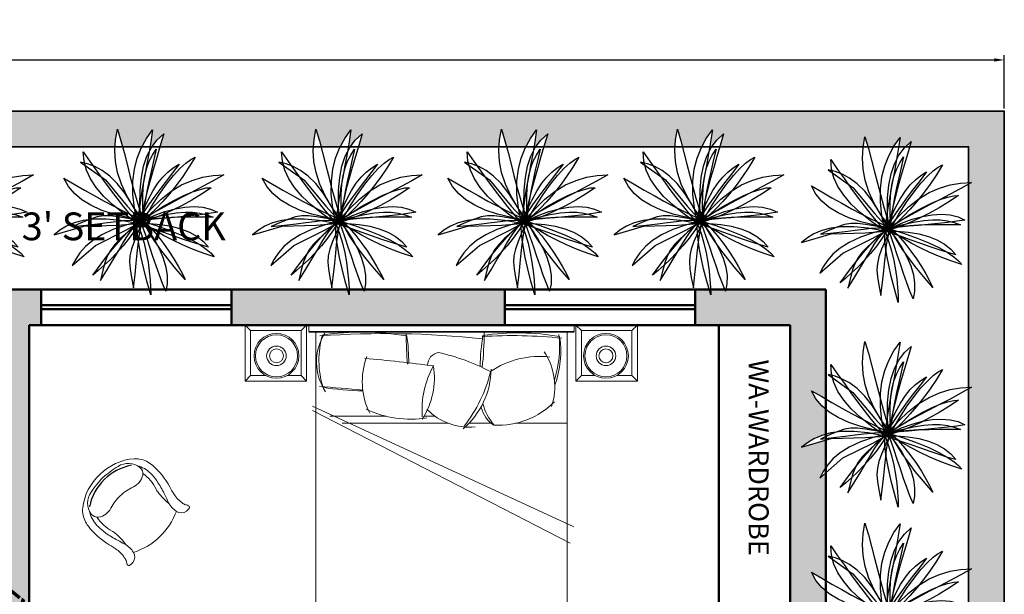
# Model space of a CAD drawing. Units: inches. Extents: x 2442 to 3851, y 589 to 2836.
# Tile 10 of 22: x 2845 to 3094, y 1880 to 2025. Entities that reach past the tile are written whole.
import ezdxf

# ---------------------------------------------------------------- set-up
doc = ezdxf.new("R2010")
doc.units = ezdxf.units.IN
for name, color, linetype, lineweight in [('0.10', 252, 'Continuous', 9), ('0.15', 34, 'Continuous', 15), ('A-ANNO-DIMS', 2, 'Continuous', 18), ('A-ANNO-TEXT', 7, 'Continuous', 18), ('A-FURN', 8, 'Continuous', 18), ('A-WALL', 7, 'Continuous', 50), ('A-WALL-PATT', 8, 'Continuous', 13), ('C-PROP', 7, 'Continuous', 35), ('L-PLNT', 94, 'Continuous', 18)]:
    doc.layers.add(name, color=color, linetype=linetype, lineweight=lineweight)
doc.layers.add('DIENHOA', color=3, linetype='Continuous')
doc.layers.add('IFF-FURN-DETAIL', color=250, linetype='Continuous')
doc.styles.get("Standard").update_dxf_attribs({"font": 'arial.ttf'})
doc.dimstyles.new('ISO-25', dxfattribs={"dimtxt": 8, "dimasz": 2.5, "dimexe": 1.25, "dimexo": 0.625, "dimtad": 1, "dimlunit": 3, "dimtxsty": 'Standard', "dimcen": 2.5, "dimadec": 0, "dimazin": 0, "dimtfac": 1, "dimtmove": 0, "dimatfit": 3, "dimfxl": 1, "dimarcsym": 0})

# ---------------------------------------------------------------- blocks, each defined once
blk = doc.blocks.new('camita')
at = {"layer": '0.10'}
for p, q in [((-0.85, -0.045), (0.85, -0.045)), ((-0.805, -0.045), (-0.805, -2.0485)), ((0.805, -0.045), (0.805, -2.0485)), ((-0.8271, -0.521), (0.8464, -1.2932)), ((-0.8271, -0.5476), (0.8236, -1.3992)), ((-0.7161, -0.585), (-0.3554, -0.585)), ((-0.638, -0.63), (0.0434, -0.63)), ((-0.1136, -0.585), (-0.0485, -0.585)), ((0.1749, -0.63), (0.3179, -0.63)), ((0.4739, -0.63), (0.805, -0.63)), ((-0.8354, -2), (0.8464, -2))]:
    blk.add_line(p, q, dxfattribs=at)
blk.add_lwpolyline([(-0.85, -0.0405), (0.85, -0.0405), (0.85, 0), (-0.85, 0)], close=True, dxfattribs=at)
for centre, radius, start, end in [((-0.4574, -0.2364), 0.3443, 147.50996, 213.83359), ((-0.3639, -5.8457), 5.7909, 83.80731, 94.12107), ((-0.5104, -1.7232), 1.6781, 80.12554, 98.66187), ((2.3534, -0.0532), 2.5803, 180.10628, 184.38541), ((-1.4396, -0.0609), 1.7117, 352.92911, 0.39592), ((0.4863, -1.6286), 1.5781, 80.16015, 98.05996), ((0.0294, -0.1377), 0.7262, 342.58415, 6.00484), ((-0.1997, -0.2266), 0.5864, 163.92635, 197.14087), ((-1.5443, -0.2452), 1.3333, 359.93941, 7.55329), ((1.5815, -0.2893), 1.3353, 170.38021, 178.99138), ((0.4524, -3.0675), 2.9996, 83.90257, 93.67595), ((0.1326, -0.1696), 0.6307, 339.92303, 8.74334), ((-0.007, -0.258), 0.0828, 100.01798, 179.73597), ((-0.2931, -1.4378), 1.2903, 61.97485, 77.84351), ((0.3203, -0.3944), 0.4043, 341.45245, 33.45121), ((-0.0543, -0.3633), 0.4542, 159.30257, 206.50263), ((-1.3301, -9.6748), 9.4985, 82.27078, 84.93989), ((0.6265, -0.7518), 0.5508, 82.96906, 124.67388), ((0.4585, -0.5454), 0.5842, 151.04555, 184.14969), ((-0.5341, -0.3393), 0.4875, 327.26442, 9.0473), ((-0.1986, -0.2742), 0.5159, 310.73945, 359.05759), ((-0.5673, -0.0868), 0.9057, 321.69527, 346.46261), ((-1.8672, -14.986), 14.6323, 84.65974, 85.75157), ((-0.4598, 1.4861), 1.9092, 260.95299, 268.65169), ((0.5707, -0.4317), 0.3145, 192.93877, 221.96363), ((0.3612, -0.133), 0.5096, 267.25889, 315.29965), ((-0.2002, 0.064), 0.6673, 244.78094, 279.06058), ((0.179, -0.272), 0.3828, 224.52836, 275.22287), ((0.4384, -0.4834), 0.1898, 193.68485, 236.70352)]:
    blk.add_arc(centre, radius, start, end, dxfattribs=at)
blk = doc.blocks.new('VELADOR')
at = {"layer": '0.15'}
for p, q in [((-0.2475, 0), (-0.2025, -0.045)), ((0.2475, 0), (0.2025, -0.045)), ((-0.2025, -0.405), (-0.2475, -0.45)), ((0.2475, -0.45), (0.2025, -0.405))]:
    blk.add_line(p, q, dxfattribs=at)
blk.add_lwpolyline([(-0.2475, 0), (-0.2475, -0.45), (0.2475, -0.45), (0.2475, 0)], close=True, dxfattribs=at)
blk.add_lwpolyline([(0.0921, -0.405), (0.2025, -0.405), (0.2025, -0.045), (-0.2025, -0.045), (-0.2025, -0.405), (-0.0818, -0.405)], dxfattribs=at)
for radius in [0.18, 0.1688, 0.0788, 0.0563]:
    blk.add_circle((0.0052, -0.2474), radius, dxfattribs=at)
blk = doc.blocks.new('ILNG95')
for points in [[(120, 308, -0.32971), (51, 384, -0.036099), (50, 422, -0.497733), (75, 439, -0.070621), (96, 429, 0.101868), (133, 414, 0.091794), (259, 412, 0.024114), (351, 433, -0.090294), (638, 458, -0.132412), (775, 407, -0.068618), (816, 368, -0.184346), (943, 0, 1.803905)], [(120, 308, 0.138132), (244, 313, 0.001085), (325, 339, -0.034227), (462, 375, -0.033255), (567, 387, -0.137428), (727, 350, -4.561553)], [(120, 308, 0.138132), (244, 313, 0.001085), (325, 339, -0.034227), (462, 375, -0.033255), (567, 387, -0.137428), (727, 350, -4.561553)], [(235, 308, 0.064243), (394, 307, 0.04414), (433, 315, -0.118032), (643, 329, -6.296816)], [(235, 308, 0.064243), (394, 307, 0.04414), (433, 315, -0.118032), (643, 329, -6.296816)], [(639, 0, 0.078302), (612, 161, -0.233633), (633, 315, -0.28763), (710, 349, -0.317923), (875, 193, -0.032882), (900, 0, 1.140397)], [(639, 0, 0.078302), (612, 161, -0.233633), (633, 315, -0.28763), (710, 349, -0.317923), (875, 193, -0.032882), (900, 0, 1.140397)], [(120, -308, 0.32971), (51, -384, 0.036099), (50, -422, 0.497733), (75, -439, 0.070621), (96, -429, -0.101868), (133, -414, -0.091794), (259, -412, -0.024114), (351, -433, 0.090294), (638, -458, 0.132412), (775, -407, 0.068618), (816, -368, 0.184346), (943, 0, -1.803905)], [(639, 0, -0.078302), (612, -161, 0.233633), (633, -315, 0.28763), (710, -349, 0.317923), (875, -193, 0.032882), (900, 0, -1.140397)], [(639, 0, -0.078302), (612, -161, 0.233633), (633, -315, 0.28763), (710, -349, 0.317923), (875, -193, 0.032882), (900, 0, -1.140397)], [(120, -308, -0.138132), (244, -313, -0.001085), (325, -339, 0.034227), (462, -375, 0.033255), (567, -387, 0.137428), (727, -350, 4.561553)], [(120, -308, -0.138132), (244, -313, -0.001085), (325, -339, 0.034227), (462, -375, 0.033255), (567, -387, 0.137428), (727, -350, 4.561553)], [(235, -308, -0.064243), (394, -307, -0.04414), (433, -315, 0.118032), (643, -329, 6.296816)], [(235, -308, -0.064243), (394, -307, -0.04414), (433, -315, 0.118032), (643, -329, 6.296816)]]:
    blk.add_lwpolyline(points, format="xyb")
blk.add_arc((759, 1), 709, 154.3281, 205.801)
at = {"layer": 'IFF-FURN-DETAIL'}
blk.add_arc((326, -2), 549, 326.8997, 34.6691, dxfattribs=at)
blk.add_arc((326, -2), 549, 326.8997, 34.6691, dxfattribs=at)
blk = doc.blocks.new('Cay03_mb')
at = {"layer": 'DIENHOA'}
for p, q in [((79.5, 503.7), (118.6, 555.3)), ((118.6, 555.3), (166.2, 599.1)), ((166.2, 599.1), (142.2, 519.4)), ((48.6, 443.6), (79.5, 503.7)), ((142.2, 519.4), (119, 441.7)), ((25.5, 374.3), (48.6, 443.6)), ((119, 441.7), (96.7, 365.6)), ((-365.2, 390.3), (-414.4, 402.8)), ((-414.4, 402.8), (-240.2, 277.8)), ((-314.9, 371.3), (-365.2, 390.3)), ((-263.5, 343.5), (-314.9, 371.3)), ((9.9, 295.3), (25.5, 374.3)), ((96.7, 365.6), (75.6, 290.6)), ((-211.2, 304.6), (-263.5, 343.5)), ((-240.2, 277.8), (-88.4, 94.9)), ((-158, 252.3), (-211.2, 304.6)), ((1.6, 205.7), (9.9, 295.3)), ((75.6, 290.6), (55.7, 216.3)), ((290.6, 243.2), (363.4, 275.4)), ((363.4, 275.4), (436.8, 297.2)), ((436.8, 297.2), (511, 309.6)), ((511, 309.6), (585.9, 313.5)), ((585.9, 313.5), (511.8, 271.4)), ((-104.2, 184.4), (-158, 252.3)), ((55.7, 216.3), (37.3, 142.1)), ((218.5, 199.8), (290.6, 243.2)), ((437.6, 231.5), (363.7, 192.9)), ((511.8, 271.4), (437.6, 231.5)), ((-49.6, 98.5), (-104.2, 184.4)), ((0.2, 104.9), (1.6, 205.7)), ((37.3, 142.1), (20.5, 67.6)), ((75.9, 75.2), (147, 144.1)), ((147, 144.1), (218.5, 199.8)), ((290.2, 154.9), (217.4, 116.6)), ((363.7, 192.9), (290.2, 154.9)), ((-88.4, 94.9), (5.4, -7.8)), ((5.4, -7.8), (-49.6, 98.5)), ((5.4, -7.8), (0.2, 104.9)), ((5.4, -7.8), (75.9, 75.2)), ((145.5, 77.3), (74.7, 36.1)), ((217.4, 116.6), (145.5, 77.3)), ((-345, 5.4), (-399.6, -17.1)), ((-298.6, 20.1), (-345, 5.4)), ((-254.7, 27.4), (-298.6, 20.1)), ((-208, 27.8), (-254.7, 27.4)), ((-152.7, 21.7), (-208, 27.8)), ((-83.4, 9.7), (-152.7, 21.7)), ((5.4, -7.8), (-83.4, 9.7)), ((20.5, 67.6), (5.4, -7.8)), ((74.7, 36.1), (5.4, -7.8)), ((5.4, -7.8), (100.3, 18.4)), ((46.3, 0.9), (5.4, -7.8)), ((96.7, 7.5), (46.3, 0.9)), ((155, 12.2), (96.7, 7.5)), ((100.3, 18.4), (182.2, 37.2)), ((219.6, 15.4), (155, 12.2)), ((182.2, 37.2), (253, 48.9)), ((289, 17.4), (219.6, 15.4)), ((253, 48.9), (314.6, 54.1)), ((361.6, 18.5), (289, 17.4)), ((314.6, 54.1), (369.2, 53.3)), ((435.8, 18.9), (361.6, 18.5)), ((369.2, 53.3), (418.6, 46.8)), ((418.6, 46.8), (464.9, 35.2)), ((510, 19), (435.8, 18.9)), ((464.9, 35.2), (510, 19)), ((-399.6, -17.1), (-468, -47.9)), ((-468, -47.9), (-375.6, -37.8)), ((-375.6, -37.8), (-295.3, -27.9)), ((-295.3, -27.9), (-225.8, -18.9)), ((-225.8, -18.9), (-165.8, -11.3)), ((-165.8, -11.3), (-114, -5.7)), ((-114, -5.7), (-69, -2.9)), ((-79.8, -79.6), (-45.1, -46.3)), ((-69, -2.9), (-29.6, -3.4)), ((-45.1, -46.3), (-16.5, -22.4)), ((5.4, -7.8), (-33.2, -69.5)), ((-29.6, -3.4), (5.4, -7.8)), ((-16.5, -22.4), (5.4, -7.8)), ((5.4, -7.8), (56.8, -73.3)), ((25.9, -64.4), (5.4, -7.8)), ((5.4, -7.8), (112.8, -40.3)), ((53.5, -41.6), (5.4, -7.8)), ((47, -125.9), (25.9, -64.4)), ((107, -75.7), (53.5, -41.6)), ((112.8, -40.3), (207.5, -73.8)), ((-165.9, -174.1), (-120.2, -122.1)), ((-120.2, -122.1), (-79.8, -79.6)), ((-74.6, -127.3), (-117.8, -181.1)), ((-33.2, -69.5), (-74.6, -127.3)), ((68.7, -190.6), (47, -125.9)), ((56.8, -73.3), (100.4, -139.1)), ((165.5, -109.6), (107, -75.7)), ((228.7, -142.8), (165.5, -109.6)), ((207.5, -73.8), (289.5, -107.6)), ((289.5, -107.6), (359.3, -141.1)), ((-216.3, -235.6), (-165.9, -174.1)), ((-117.8, -181.1), (-162.1, -230.9)), ((90.8, -256.6), (68.7, -190.6)), ((100.4, -139.1), (135.9, -204.3)), ((135.9, -204.3), (162.8, -268.3)), ((296, -174.7), (228.7, -142.8)), ((367.1, -204.8), (296, -174.7)), ((359.3, -141.1), (416.9, -173.5)), ((441.6, -232.7), (367.1, -204.8)), ((416.9, -173.5), (462.6, -204.2)), ((462.6, -204.2), (496.5, -232.5)), ((-271, -306.6), (-216.3, -235.6)), ((-162.1, -230.9), (-206.3, -276.5)), ((113.1, -322.2), (90.8, -256.6)), ((162.8, -268.3), (181, -330.4)), ((518.9, -257.7), (441.6, -232.7)), ((496.5, -232.5), (518.9, -257.7)), ((-329.5, -387.1), (-271, -306.6)), ((-249.6, -317.8), (-291, -354.7)), ((-206.3, -276.5), (-249.6, -317.8)), ((135.4, -385.6), (113.1, -322.2)), ((181, -330.4), (190, -390)), ((-291, -354.7), (-329.5, -387.1)), ((157.6, -445), (135.4, -385.6)), ((190, -390), (189.6, -446.3)), ((179.5, -498.7), (157.6, -445)), ((189.6, -446.3), (179.5, -498.7))]:
    blk.add_line(p, q, dxfattribs=at)
for points in [[(23.7, -5.4), (-41, 82.2), (-91.8, 167.1), (-129.7, 249.5), (-155.6, 329.6), (-170.2, 407.8), (-174.7, 484.2), (-169.8, 559.3), (-156.5, 633.1)], [(-156.5, 633.1), (-132.5, 551.3), (-110.5, 470), (-89.8, 389.2), (-69.6, 309), (-49, 229.4), (-27.1, 150.4), (-3.2, 72.1), (23.7, -5.4)], [(-16.4, -26.7), (-38.3, 80), (-48.9, 178.3), (-48.7, 269), (-38.5, 352.6), (-19.1, 429.7), (9, 501), (44.9, 567.1), (87.9, 628.5)], [(87.9, 628.5), (75.5, 544.2), (61.3, 461.2), (46.1, 379.1), (30.8, 297.8), (16.1, 216.9), (2.9, 136), (-8.3, 54.9), (-16.4, -26.7)], [(23.7, -5.4), (19.8, 93), (20.3, 177), (25, 248.5), (34, 309.8), (47.3, 362.7), (64.9, 409.3), (86.8, 451.7), (112.9, 491.9)], [(112.9, 491.9), (96, 419.7), (79.5, 347.4), (63.9, 276.5), (50, 208.4), (38.4, 144.8), (29.7, 86.9), (24.6, 36.3), (23.7, -5.4)], [(-395.6, 473.7), (-347.5, 405.6), (-300.6, 339.5), (-254.3, 275.1), (-208.3, 212.3), (-161.9, 150.9), (-114.8, 90.7), (-66.5, 31.6), (-16.4, -26.7)], [(-16.4, -26.7), (-108.3, 38.6), (-186.9, 101.7), (-252.4, 163.5), (-305.1, 224.4), (-345.4, 285.2), (-373.7, 346.6), (-390.4, 409.2), (-395.6, 473.7)], [(384.3, 437.5), (342.2, 367.8), (298.1, 301.7), (252.6, 239.4), (206.1, 181.1), (159.4, 127.2), (113, 78), (67.6, 33.6), (23.7, -5.4)], [(23.7, -5.4), (79.9, 91.7), (134.1, 176.2), (185.8, 248.4), (234.3, 308.7), (279, 357.3), (319.3, 394.8), (354.6, 421.4), (384.3, 437.5)], [(273.2, 387.3), (227.6, 328.8), (182.3, 270.1), (138.4, 212.3), (97.2, 156.4), (60, 103.4), (27.8, 54.6), (1.9, 10.8), (-16.4, -26.7)], [(-16.4, -26.7), (21.4, 64.2), (57, 140.3), (91.4, 203.3), (125.2, 255.1), (159.5, 297.5), (195, 332.5), (232.7, 361.8), (273.2, 387.3)], [(-530.5, 289.7), (-458.3, 248.1), (-387.9, 207.8), (-318.9, 168.7), (-250.8, 131.1), (-182.9, 94.8), (-114.9, 59.9), (-46.2, 26.5), (23.7, -5.4)], [(23.7, -5.4), (-87.2, 15.2), (-185, 39.6), (-270.3, 68.2), (-343.7, 101.4), (-405.9, 139.7), (-457.3, 183.5), (-498.7, 233.4), (-530.5, 289.7)], [(496.7, 224), (429.4, 178.4), (361.6, 136.9), (294.1, 99.5), (227.5, 66.1), (162.4, 36.7), (99.7, 11.5), (39.8, -9.7), (-16.4, -26.7)], [(-16.4, -26.7), (75.4, 37.9), (160.1, 91.8), (237.3, 135.7), (306.6, 170), (367.6, 195.4), (419.9, 212.5), (463.1, 221.9), (496.7, 224)], [(23.7, -5.4), (99.3, 29.7), (173.2, 57.1), (244.8, 76.7), (313.3, 88.3), (377.9, 91.8), (437.9, 87), (492.7, 73.8), (541.4, 52)], [(-16.4, -26.7), (-134, -4.7), (-235.3, 5.3), (-322, 4.7), (-395.9, -5), (-458.7, -22.3), (-512.3, -45.7), (-558.2, -73.6), (-598.4, -104.7)], [(541.4, 52), (484.1, 42.9), (421.2, 34.8), (354.4, 27.6), (285.4, 20.9), (216.1, 14.5), (148.2, 8.1), (83.5, 1.6), (23.7, -5.4)], [(-598.4, -104.7), (-392.7, -44.4), (-155, -37.4), (-16.4, -26.7)], [(-471.9, -320.3), (-310.5, -179.3), (-97.7, -73.3), (23.7, -5.4)], [(23.7, -5.4), (-92.3, -34.8), (-188.4, -68.2), (-266.9, -105.1), (-329.9, -144.9), (-379.7, -187), (-418.5, -230.7), (-448.5, -275.3), (-471.9, -320.3)], [(-276.2, -424.4), (-227.3, -345.4), (-185.7, -276.1), (-150, -215.7), (-119.1, -163.8), (-91.5, -119.5), (-66, -82.3), (-41.4, -51.6), (-16.4, -26.7)], [(-16.4, -26.7), (-84.9, -86), (-137, -133.1), (-175.8, -173), (-204.3, -210), (-225.5, -249.1), (-242.5, -294.7), (-258.4, -351.6), (-276.2, -424.4)], [(23.7, -5.4), (-13.6, -87.9), (-41.1, -152.6), (-59.6, -205), (-69.9, -250.7), (-72.8, -295), (-69.2, -343.6), (-59.7, -401.9), (-45.3, -475.5)], [(-45.3, -475.5), (-34.1, -383.2), (-25.4, -302.8), (-18.3, -233.1), (-12, -172.9), (-5.6, -121.2), (2, -76.8), (11.4, -38.5), (23.7, -5.4)], [(76.2, -524.2), (48.8, -428.5), (26.6, -341.7), (9.2, -264.1), (-3.6, -196.1), (-12.3, -138), (-17.1, -90.2), (-18.3, -53), (-16.4, -26.7)], [(-16.4, -26.7), (66.9, -26.6), (145.6, -32.7), (218.8, -44.9), (285.8, -63.1), (345.9, -87.1), (398.4, -116.6), (442.6, -151.6), (477.6, -191.8)], [(477.6, -191.8), (421.8, -176), (361.3, -156.9), (297.6, -135.5), (232.2, -112.6), (166.6, -89.4), (102.3, -66.6), (40.8, -45.4), (-16.4, -26.7)], [(-16.4, -26.7), (8.5, -95.1), (28.5, -163.3), (44.3, -230.6), (56.3, -296.1), (65, -359), (70.9, -418.5), (74.5, -473.9), (76.2, -524.2)], [(316.5, -418.1), (251.4, -342.8), (194.8, -273.3), (146.5, -210.2), (106.3, -153.8), (74.1, -104.7), (49.7, -63.4), (32.9, -30.1), (23.7, -5.4)], [(23.7, -5.4), (74.9, -57.1), (121.8, -110.6), (164.3, -165), (202.7, -219.4), (237, -272.9), (267.3, -324.5), (293.7, -373.2), (316.5, -418.1)]]:
    blk.add_lwpolyline(points, dxfattribs=at)
blk = doc.blocks.new('*D31')
at = {"layer": 'A-ANNO-DIMS', "color": 0, "lineweight": -2, "transparency": 16777216}
for p, q in [((2493.6, 2002.49), (2493.6, 2016.02)), ((2496.1, 2014.77), (3091.1, 2014.77)), ((3093.6, 2002.49), (3093.6, 2016.02))]:
    blk.add_line(p, q, dxfattribs=at)
at = {"layer": 'A-ANNO-DIMS', "color": 0, "transparency": 16777216}
for points in [[(2496.1, 2015.19), (2496.1, 2014.36), (2493.6, 2014.77)], [(3091.1, 2015.19), (3091.1, 2014.36), (3093.6, 2014.77)]]:
    blk.add_solid(points, dxfattribs=at)
at = {"layer": 'Defpoints', "color": 0, "transparency": 16777216}
for p in [(3093.6, 2014.77), (2493.6, 2001.86), (3093.6, 2001.86)]:
    blk.add_point(p, dxfattribs=at)
at = {"layer": 'A-ANNO-DIMS', "color": 0, "transparency": 16777216, "insert": (2793.6, 2019.48), "char_height": 8, "attachment_point": 5}
blk.add_mtext("50'", dxfattribs=at)
blk = doc.blocks.new('*D144')
at = {"layer": 'A-ANNO-DIMS', "color": 0, "lineweight": -2, "transparency": 16777216}
for p, q in [((2857.1, 1857.27), (2728.92, 1961.48)), ((2858.85, 1859.43), (2856.31, 1856.3)), ((2872.8, 1844.49), (2859.04, 1855.69)), ((2876.5, 1845.08), (2873.96, 1841.94))]:
    blk.add_line(p, q, dxfattribs=at)
at = {"layer": 'A-ANNO-DIMS', "color": 0, "transparency": 16777216}
for points in [[(2859.3, 1856.01), (2858.77, 1855.36), (2857.1, 1857.27)], [(2873.07, 1844.82), (2872.54, 1844.17), (2874.74, 1842.91)]]:
    blk.add_solid(points, dxfattribs=at)
at = {"layer": 'Defpoints', "color": 0, "transparency": 16777216}
for p in [(2859.25, 1859.91), (2857.1, 1857.27), (2876.9, 1845.56)]:
    blk.add_point(p, dxfattribs=at)
at = {"layer": 'A-ANNO-DIMS', "color": 0, "transparency": 16777216, "insert": (2795.04, 1913.86), "char_height": 8, "attachment_point": 5, "rotation": 320.8857}
blk.add_mtext('LOUNGE CHAIR 1\'-10 1/2" TYP.', dxfattribs=at)

msp = doc.modelspace()

# ---------------------------------------------------------------- hatches: boundary and pattern name
at = {"layer": 'A-WALL-PATT'}
h = msp.add_hatch(color=256, dxfattribs=at)
h.dxf.hatch_style = 1
h.paths.add_polyline_path([(2502.599, 1992.864), (2719.571, 1992.864), (2719.687, 1994.649), (2720.167, 1997.319), (2721.479, 1992.864), (2726.325, 1992.864), (2727.448, 1994.93), (2729.005, 1997.153), (2728.372, 1992.864), (2728.871, 1992.864), (2730.114, 1994.505), (2731.833, 1996.09), (2730.966, 1993.206), (2730.864, 1992.864), (2771.772, 1992.864), (2771.887, 1994.649), (2772.368, 1997.319), (2773.68, 1992.864), (2778.526, 1992.864), (2779.649, 1994.93), (2781.206, 1997.153), (2780.572, 1992.864), (2781.072, 1992.864), (2782.315, 1994.505), (2784.034, 1996.09), (2783.167, 1993.206), (2783.065, 1992.864), (2821.282, 1992.864), (2821.398, 1994.649), (2821.878, 1997.319), (2823.19, 1992.864), (2828.036, 1992.864), (2829.159, 1994.93), (2830.716, 1997.153), (2830.083, 1992.864), (2830.582, 1992.864), (2831.825, 1994.505), (2833.544, 1996.09), (2832.677, 1993.206), (2832.575, 1992.864), (2869.287, 1992.864), (2869.403, 1994.649), (2869.884, 1997.319), (2871.195, 1992.864), (2876.042, 1992.864), (2877.165, 1994.93), (2878.721, 1997.153), (2878.088, 1992.864), (2878.587, 1992.864), (2879.83, 1994.505), (2881.55, 1996.09), (2880.682, 1993.206), (2880.58, 1992.864), (2919.335, 1992.864), (2919.451, 1994.649), (2919.932, 1997.319), (2921.243, 1992.864), (2926.09, 1992.864), (2927.213, 1994.93), (2928.77, 1997.153), (2928.136, 1992.864), (2928.635, 1992.864), (2929.878, 1994.505), (2931.598, 1996.09), (2930.73, 1993.206), (2930.628, 1992.864), (2966.155, 1992.864), (2966.27, 1994.649), (2966.751, 1997.319), (2968.063, 1992.864), (2972.909, 1992.864), (2974.032, 1994.93), (2975.589, 1997.153), (2974.955, 1992.864), (2975.455, 1992.864), (2976.698, 1994.505), (2978.417, 1996.09), (2977.55, 1993.206), (2977.448, 1992.864), (3010.53, 1992.864), (3010.646, 1994.649), (3011.127, 1997.319), (3012.438, 1992.864), (3017.285, 1992.864), (3018.408, 1994.93), (3019.964, 1997.153), (3019.331, 1992.864), (3019.83, 1992.864), (3021.073, 1994.505), (3022.793, 1996.09), (3021.925, 1993.206), (3021.823, 1992.864), (3057.996, 1992.864), (3058.45, 1995.382), (3059.191, 1992.864), (3065.64, 1992.864), (3067.287, 1995.216), (3066.94, 1992.864), (3068.717, 1992.864), (3070.116, 1994.153), (3069.728, 1992.864), (3084.599, 1992.864), (3084.599, 1983.791), (3085.291, 1983.828), (3084.599, 1983.434), (3084.599, 1932.114), (3085.291, 1932.151), (3084.599, 1931.757), (3084.599, 1886.278), (3085.291, 1886.315), (3084.599, 1885.921), (3084.599, 1410.864), (3066.599, 1410.864), (3066.599, 1401.864), (3093.599, 1401.864), (3093.599, 2001.864), (2493.599, 2001.864), (2493.599, 1401.864), (2538.599, 1401.864), (2538.599, 1410.864), (2502.599, 1410.864)])
h.paths.add_polyline_path([(2738.599, 1410.864), (2547.599, 1410.864), (2547.599, 1401.864), (2738.599, 1401.864)], flags=17)
h.paths.add_polyline_path([(2910.599, 1410.864), (2792.599, 1410.864), (2792.599, 1401.864), (2910.599, 1401.864), (2910.599, 1402.864)], flags=17)
h = msp.add_hatch(color=256, dxfattribs=at)
h.dxf.hatch_style = 1
h.paths.add_polyline_path([(2799.599, 1467.864), (2775.599, 1467.864), (2775.599, 1458.864), (2799.599, 1458.864)])
h.paths.add_polyline_path([(2703.599, 1506.864), (2670.599, 1506.864), (2670.599, 1497.864), (2694.599, 1497.864), (2694.599, 1458.864), (2733.599, 1458.864), (2733.599, 1467.864), (2709.417, 1467.864), (2703.599, 1467.864)])
h.paths.add_polyline_path([(2604.599, 1506.864), (2593.599, 1506.864), (2593.599, 1497.864), (2604.599, 1497.864)])
h.paths.add_polyline_path([(2547.599, 1497.864), (2553.599, 1497.864), (2553.599, 1506.864), (2547.599, 1506.864), (2547.599, 1530.864), (2538.599, 1530.864), (2538.599, 1401.864), (2547.599, 1401.864)])
h.paths.add_polyline_path([(2547.599, 1683.864), (2538.599, 1683.864), (2538.599, 1578.864), (2547.599, 1578.864), (2547.599, 1602.864), (2694.599, 1602.864), (2694.599, 1554.864), (2703.599, 1554.864), (2703.599, 1716.864), (2694.599, 1716.864), (2694.599, 1611.864), (2547.599, 1611.864)])
h.paths.add_polyline_path([(2892.599, 1497.864), (2883.599, 1497.864), (2883.599, 1488.228), (2883.599, 1467.864), (2865.599, 1467.864), (2865.599, 1458.864), (2892.599, 1458.864)])
h.paths.add_polyline_path([(3048.599, 1722.864), (3039.599, 1722.864), (3039.599, 1716.864), (2937.599, 1716.864), (2937.599, 1710.864), (3039.599, 1710.864), (3039.599, 1685.364), (3048.599, 1685.364)])
h.paths.add_polyline_path([(3048.599, 1779.864), (3039.599, 1779.864), (3039.599, 1773.864), (2961.599, 1773.864), (2961.599, 1791.864), (2955.599, 1791.864), (2955.599, 1773.864), (2895.599, 1773.864), (2895.599, 1821.864), (2916.599, 1821.864), (2916.599, 1827.864), (2889.599, 1827.864), (2889.599, 1773.864), (2886.599, 1773.864), (2886.599, 1764.864), (2937.599, 1764.864), (2937.599, 1746.864), (2943.599, 1746.864), (2943.599, 1764.864), (2956.06, 1764.864), (3039.599, 1764.864), (3039.599, 1758.864), (3048.599, 1758.864)])
h.paths.add_polyline_path([(3048.599, 1827.864), (2976.475, 1827.864, -0.1284593), (2975.705, 1827.665), (2964.694, 1827.687, -0.1198794), (2963.972, 1827.864), (2946.599, 1827.864), (2946.599, 1821.864), (3039.599, 1821.864), (3039.599, 1815.864), (3048.599, 1815.864)])
h.paths.add_polyline_path([(3048.599, 1956.864), (3023.366, 1956.864), (3023.277, 1956.402), (3023.088, 1956.864), (3019.494, 1956.864), (3019.543, 1955.479), (3019.146, 1956.864), (3015.599, 1956.864), (3015.599, 1947.864), (3039.599, 1947.864), (3039.599, 1875.864), (3048.599, 1875.864), (3048.599, 1880.743), (3047.576, 1881.614), (3046.081, 1883.417), (3044.931, 1885.453), (3047.541, 1883.949), (3048.599, 1883.343), (3048.599, 1910.588), (3047.049, 1909.235), (3047.896, 1910.862), (3048.599, 1911.909), (3048.599, 1918.826), (3042.477, 1917.032), (3043.928, 1918.154), (3045.59, 1919.165), (3047.525, 1920.009), (3048.599, 1920.305), (3048.599, 1926.579), (3047.576, 1927.45), (3046.081, 1929.252), (3044.931, 1931.289), (3047.541, 1929.785), (3048.599, 1929.179)])
h.paths.add_polyline_path([(2967.599, 1956.864), (2932.171, 1956.864), (2932.082, 1956.402), (2931.893, 1956.864), (2928.299, 1956.864), (2928.348, 1955.479), (2927.951, 1956.864), (2898.599, 1956.864), (2898.599, 1947.864), (2967.599, 1947.864)])
h.paths.add_polyline_path([(2850.599, 1956.864), (2834.118, 1956.864), (2834.029, 1956.402), (2833.84, 1956.864), (2830.245, 1956.864), (2830.294, 1955.479), (2829.897, 1956.864), (2796.599, 1956.864), (2796.599, 1947.864), (2799.599, 1947.864), (2838.599, 1947.864), (2838.599, 1827.864), (2835.599, 1827.864), (2835.599, 1824.864), (2835.599, 1818.864), (2838.599, 1818.864), (2838.599, 1764.864), (2850.599, 1764.864), (2850.599, 1770.864), (2850.599, 1773.864), (2847.599, 1773.864), (2847.599, 1947.864), (2850.599, 1947.864)])
h.paths.add_polyline_path([(2700.599, 1947.864), (2730.599, 1947.864), (2730.599, 1956.864), (2700.599, 1956.864), (2700.599, 1992.864), (2691.599, 1992.864), (2691.599, 1932.864), (2670.599, 1932.864), (2670.599, 1923.864), (2691.599, 1923.864), (2691.599, 1818.864), (2799.599, 1818.864), (2799.599, 1827.864), (2700.599, 1827.864)])
h.paths.add_polyline_path([(2640.599, 1932.864), (2538.599, 1932.864), (2538.599, 1868.364), (2547.599, 1868.364), (2547.599, 1923.864), (2640.599, 1923.864), (2640.599, 1929.864)])
h.paths.add_polyline_path([(2547.599, 1820.364), (2538.599, 1820.364), (2538.599, 1731.864), (2547.599, 1731.864), (2547.599, 1755.864), (2694.599, 1755.864), (2694.599, 1752.864), (2697.599, 1752.864), (2703.599, 1752.864), (2703.599, 1764.864), (2547.599, 1764.864)])
h.paths.add_polyline_path([(2725.858, 1838.187), (2790.115, 1838.187), (2790.115, 1868.602), (2725.858, 1868.602)], flags=25)
h.paths.add_polyline_path([(2892.599, 1671.864), (2883.599, 1671.864), (2883.599, 1563.864), (2892.599, 1563.864), (2892.599, 1602.864), (3048.599, 1602.864), (3048.599, 1637.364), (3039.599, 1637.364), (3039.599, 1611.864), (2892.599, 1611.864)])

# ---------------------------------------------------------------- linework, layer by layer
at = {"layer": 'A-WALL'}
for p, q in [((2700.599, 1956.864), (3048.599, 1956.864)), ((2850.599, 1947.864), (2850.599, 1956.864)), ((2898.599, 1947.864), (2898.599, 1956.864)), ((2967.599, 1947.864), (2967.599, 1956.864)), ((3015.599, 1947.864), (3015.599, 1956.864)), ((3048.599, 1602.864), (3048.599, 1956.864)), ((2850.599, 1952.864), (2898.599, 1952.864)), ((2967.599, 1952.864), (3015.599, 1952.864)), ((2850.599, 1951.864), (2898.599, 1951.864)), ((2967.599, 1951.864), (3015.599, 1951.864)), ((2847.599, 1773.864), (2847.599, 1947.864)), ((2847.599, 1947.864), (3039.599, 1947.864)), ((3021.599, 1827.864), (3021.599, 1947.864)), ((3039.599, 1827.864), (3039.599, 1947.864))]:
    msp.add_line(p, q, dxfattribs=at)
at = {"layer": 'C-PROP'}
for points in [[(3066.599, 1401.864), (3093.599, 1401.864), (3093.599, 2001.864), (2493.599, 2001.864), (2493.599, 1401.864), (2738.599, 1401.864)], [(3066.599, 1410.864), (3084.599, 1410.864), (3084.599, 1992.864), (2502.599, 1992.864), (2502.599, 1410.864), (2538.599, 1410.864)]]:
    msp.add_lwpolyline(points, dxfattribs=at)

# ---------------------------------------------------------------- block references
at = {"layer": 'A-FURN'}
for name, p, xscale, yscale, zscale in [('VELADOR', (2909.821, 1947.864), 31.41542173157097, 31.41542173157097, 31.41542173157097), ('camita', (2951.652, 1947.864), 39.375, 39.375, 39.375)]:
    msp.add_blockref(name, p, dxfattribs=dict(at, xscale=xscale, yscale=yscale, zscale=zscale))
for name, p, xscale, yscale, zscale, rotation in [('VELADOR', (2993.27, 1947.864), -31.41542173157097, 31.41542173157097, 31.41542173157097, 359.9999999999999), ('ILNG95', (2881.345, 1893.529), 0.0243705291132055, 0.0243705291132055, 0.0243705291132055, 133.7094105413398)]:
    msp.add_blockref(name, p, dxfattribs=dict(at, xscale=xscale, yscale=yscale, zscale=zscale, rotation=rotation))
at = {"layer": 'L-PLNT', "xscale": 0.036152509973097, "yscale": 0.036152509973097, "zscale": 0.036152509973097}
for p in [(2827.538, 1974.43), (2875.543, 1974.43), (2925.591, 1974.43), (2972.411, 1974.43), (3016.786, 1974.43), (3064.109, 1972.493), (3064.109, 1920.816), (3064.109, 1874.98)]:
    msp.add_blockref('Cay03_mb', p, dxfattribs=at)

# ---------------------------------------------------------------- texts
at = {"layer": 'A-ANNO-TEXT', "insert": (2845.713, 1976.271), "char_height": 7, "attachment_point": 1}
msp.add_mtext_dynamic_manual_height_columns("{\\fTimes New Roman|b0|i0|c0|p18;3' SETBACK}", width=79.56037, gutter_width=12.5, heights=[0], dxfattribs=at)
at = {"layer": 'A-ANNO-TEXT', "insert": (3034.144, 1939.175), "char_height": 5, "attachment_point": 1, "rotation": 270}
msp.add_mtext_dynamic_manual_height_columns('{\\fTimes New Roman|b0|i0|c0|p18;WA-WARDROBE}', width=110.76054, gutter_width=12.5, heights=[0], dxfattribs=at)

# ---------------------------------------------------------------- dimensions: what is measured, and where the dimension line sits
at = {"layer": 'A-ANNO-DIMS'}
dim = msp.add_linear_dim(base=(3093.599, 2014.775), p1=(2493.599, 2001.864), p2=(3093.599, 2001.864), dimstyle='ISO-25', override={"dimclrd": 0, "dimclre": 0, "dimclrt": 0}, dxfattribs=at)
dim.commit()
dim.dimension.update_dxf_attribs({"geometry": '*D31', "text_midpoint": (2793.599, 2019.485)})
dim = msp.add_linear_dim(base=(2857.095, 1857.265), p1=(2876.897, 1845.562), p2=(2859.248, 1859.913), angle=140.88565, text='LOUNGE CHAIR <> TYP.', dimstyle='ISO-25', override={"dimdec": 1, "dimrnd": 0, "dimzin": 1, "dimlunit": 4, "dimfrac": 2}, dxfattribs=at)
dim.commit()
dim.dimension.update_dxf_attribs({"geometry": '*D144', "text_midpoint": (2795.044, 1913.859)})

doc.saveas('drawing.dxf')
